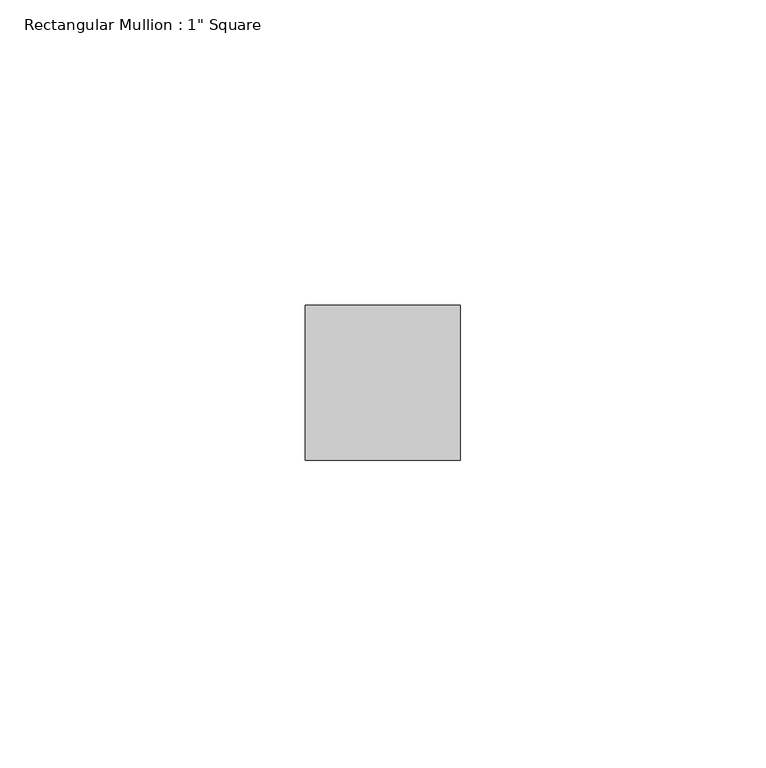
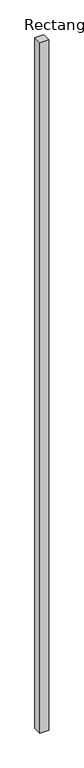
"""IFC4 building model written with IfcOpenShell, lengths in millimetres: member geometry."""

from ifc_helpers import new_model, si_unit, frame, origin, place, context, project, spatial, polyline, outline, extrude, source, transform, mapped, element, save


def member_b561e846(model_context):
    return source(origin(), model_context, "Body", "SweptSolid", [
        extrude(outline(polyline([(12.7, 12.7), (12.7, -12.7), (-12.7, -12.7), (-12.7, 12.7), (12.7, 12.7)])), frame((0.0, 0.0, -2133.6), z_axis=(0.0, 0.0, 1.0), x_axis=(1.0, 0.0, 0.0)), (0.0, 0.0, 1.0), 2133.6),
    ])


if __name__ == "__main__":
    model = new_model("IFC4")
    model_context = context("Model", 3, world=origin())
    ifc_project = project(units=[si_unit("LENGTHUNIT", "METRE", prefix="MILLI")], contexts=[model_context])
    site = spatial("IfcSite", under=ifc_project)
    building = spatial("IfcBuilding", under=site)
    placement = place(None, origin())
    member_shape = member_b561e846(model_context)
    element("IfcMember", 1, ObjectType="Rectangular Mullion : 1\" Square", at=placement, inside=building, context=model_context, shape_type="MappedRepresentation", body=[
        mapped(member_shape, transform((0.0, 0.0, 0.0), x_axis=(1.0, 0.0, 0.0), y_axis=(0.0, 1.0, 0.0), z_axis=(0.0, 0.0, 1.0))),
    ])
    save(model, "model.ifc")

# Revit data of these elements
# Type "Rectangular Mullion : 1\" Square"
#   built-in parameter 1007304 = 0.0833333 (stored number, unit not read)
#   built-in parameter 1007301 = 0.0416667 (stored number, unit not read)
#   built-in parameter 1007300 = 0.0416667 (stored number, unit not read)
# Element 1 (IfcMember, "Rectangular Mullion : 1\" Square")
#   Materials on its faces: "Aluminum"
# Materials
#   "Aluminum": class "Metal", colour RGB 247 247 247, transparency 0, Description = "Aluminum 6061", Cost = 0
